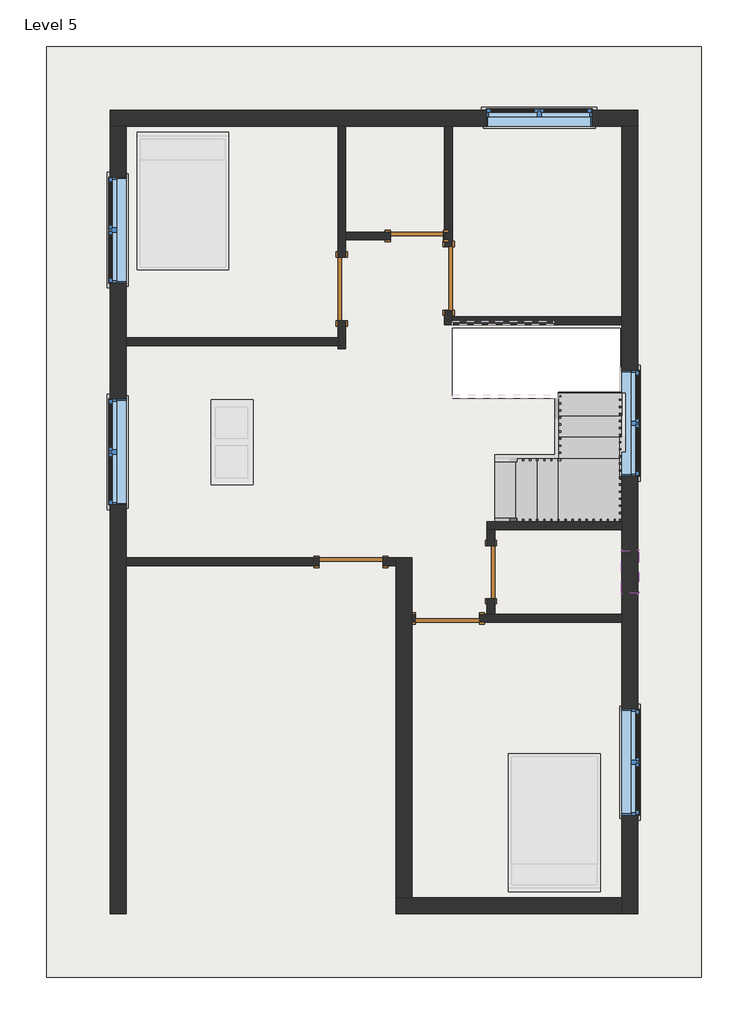
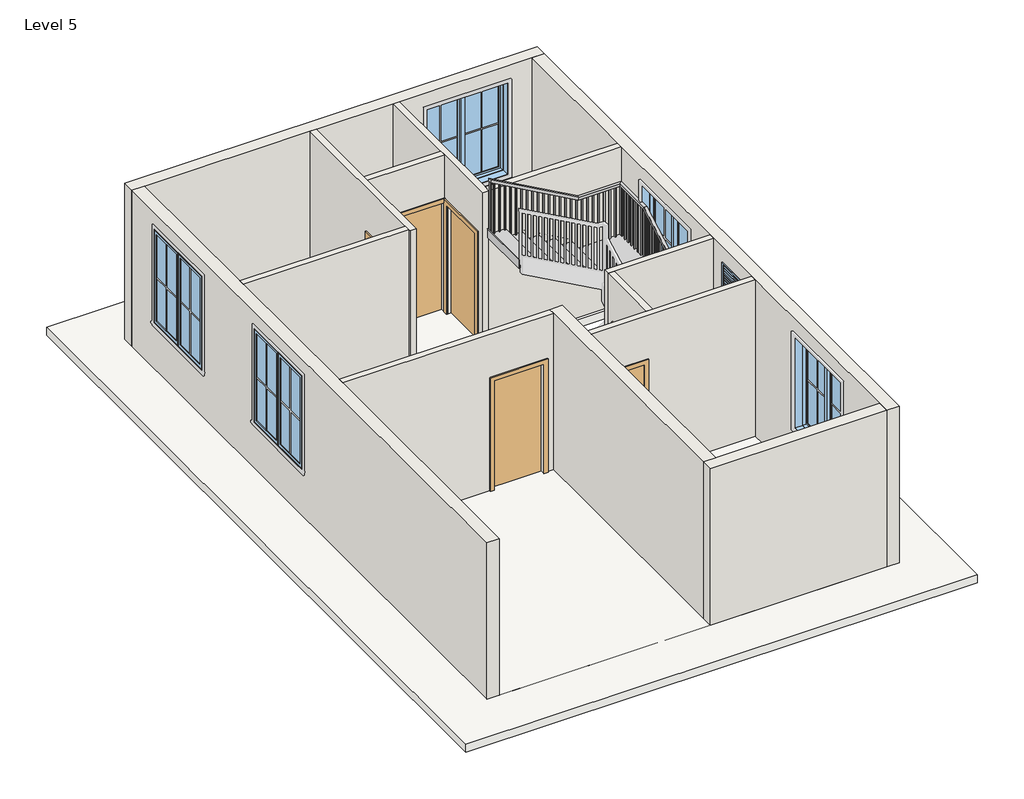
# One storey, part 1 of 2: 14 walls, 6 doors, 6 windows, 1 railing, 1 roof, 1 slab, 1 stair flight.
# Revit data of these elements (continued)
# Element 27 (IfcWindow, "Window-Casement-Double : WIN 5'")
#   Mark = "21"
#   Window Inset = 0' - 0"
#   Interior Wall Closure = 0' - 2 1/4"
#   Frame Extension = 0' - 0 1/4"
#   Exterior Wall Closure = 0' - 1 1/4"
#   Interior Trim Visibility = yes
#   Exterior Trim Visibility = yes
#   Phase Created = New Construction
#   Materials on its faces: "Wood - Stained", "Glass", "Clad - White"
# Element 28 (IfcWindow, "Window-Casement-Double : WIN 5'")
#   Mark = "22"
#   Window Inset = 0' - 0"
#   Interior Wall Closure = 0' - 2 1/4"
#   Frame Extension = 0' - 0 1/4"
#   Exterior Wall Closure = 0' - 1 1/4"
#   Interior Trim Visibility = yes
#   Exterior Trim Visibility = yes
#   Phase Created = New Construction
#   Materials on its faces: "Wood - Stained", "Glass", "Clad - White"
# Element 29 (IfcWindow, "Window-Casement-Double : WIN 5'")
#   Mark = "23"
#   Window Inset = 0' - 0"
#   Interior Wall Closure = 0' - 2 1/4"
#   Frame Extension = 0' - 0 1/4"
#   Exterior Wall Closure = 0' - 1 1/4"
#   Interior Trim Visibility = yes
#   Exterior Trim Visibility = yes
#   Phase Created = New Construction
#   Materials on its faces: "Wood - Stained", "Glass", "Clad - White"
# Element 30 (IfcWindow, "Window-Louvers : 24\" x 24\"")
#   Mark = "24"
#   Blade Width = 1' - 10 1/2"
#   Phase Created = New Construction
#   Materials on its faces: "Birch"
# Materials
#   "Door - Panel": class "Wood", colour RGB 210 159 95, transparency 0, Cost = 0
#   "Door - Frame": colour RGB 118 70 51, transparency 0, Cost = 0
#   "Wood - Stained": class "Wood", colour RGB 224 178 126, transparency 0, Cost = 0
#   "Glass": class "Glass", colour RGB 0 128 192, transparency 0.75, Description = "Soda Lime Glass", Cost = 0
#   "Clad - White": class "Wood", colour RGB 242 242 238, transparency 0, Cost = 0
#   "Birch": class "Wood", colour RGB 224 178 126, transparency 0, Description = "Betula Alleghaniensis", Cost = 0
#   "Default Roof": colour RGB 88 101 114, transparency 0, Cost = 0
#   "Default Floor": colour RGB 128 128 128, transparency 0, Cost = 0
#   "Default Wall": colour RGB 128 128 128, transparency 0, Cost = 0
#   "Copper": class "Metal", colour RGB 0 0 0, transparency 0, Description = "Copper, matte finish", Cost = 0
